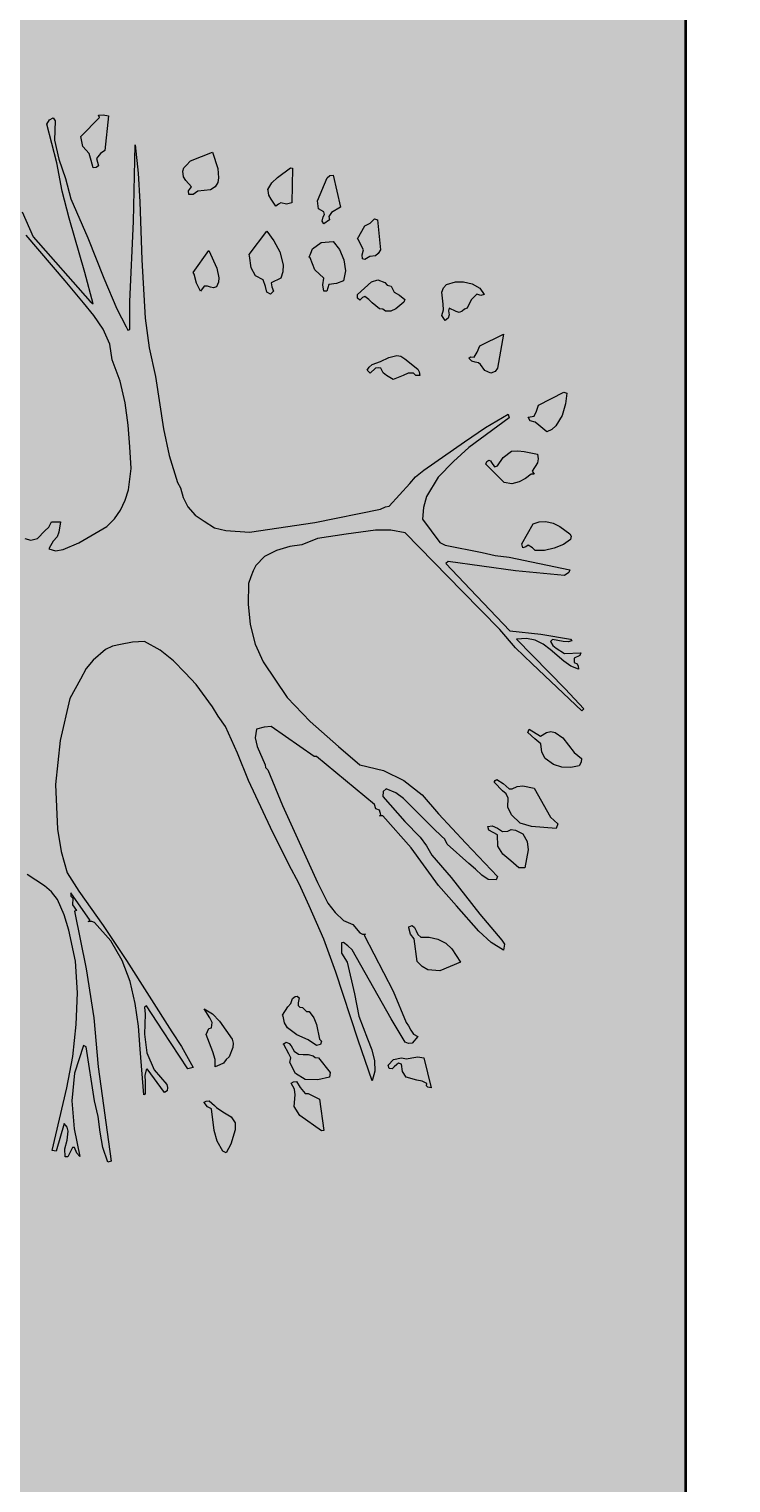
# Model space of a CAD drawing. Units: inches. Extents: x 84 to 1044, y -280 to 906.
# Tile 102 of 105: x 882 to 897, y 478 to 510. Entities that reach past the tile are written whole.
import ezdxf

# ---------------------------------------------------------------- set-up
doc = ezdxf.new("R2010")
doc.units = ezdxf.units.IN
for name, color, linetype, lineweight in [('A-ANNO-DIMS', 2, 'Continuous', 18), ('L-PLNT', 114, 'Continuous', 15), ('WALL', 250, 'Continuous', 35)]:
    doc.layers.add(name, color=color, linetype=linetype, lineweight=lineweight)
doc.layers.add('L-PLNT-PATT', color=9, linetype='Continuous', lineweight=9, true_color=0xafd9aa)
doc.styles.get("Standard").update_dxf_attribs({"font": 'arial.ttf'})
doc.dimstyles.get("Standard").update_dxf_attribs({"dimtxt": 0.18, "dimasz": 0.18, "dimexe": 0.18, "dimexo": 0.0625, "dimgap": 0.09, "dimtad": 0, "dimtih": 1, "dimtoh": 1, "dimdec": 4, "dimzin": 0, "dimdsep": 46, "dimtxsty": 'Standard', "dimcen": 0.09, "dimadec": 0, "dimazin": 0, "dimtfac": 1, "dimtdec": 4, "dimtofl": 0, "dimtmove": 0, "dimatfit": 3, "dimfxl": 1, "dimtolj": 1, "dimtzin": 0, "dimarcsym": 0})

# ---------------------------------------------------------------- blocks, each defined once
blk = doc.blocks.new('A$C37E508DF')
for p, q in [((0.7083, 1.5239), (0.7152, 1.5244)), ((0.7096, 1.5209), (0.7083, 1.5239)), ((0.7152, 1.5244), (0.7225, 1.5231)), ((0.6329, 1.5111), (0.6367, 1.5175)), ((0.6475, 1.4545), (0.6329, 1.5111)), ((0.6367, 1.5175), (0.6423, 1.5201)), ((0.6423, 1.5201), (0.6453, 1.5158)), ((0.6453, 1.5158), (0.644, 1.4879)), ((0.6826, 1.493), (0.7096, 1.5209)), ((0.7225, 1.5231), (0.7174, 1.4729)), ((0.644, 1.4879), (0.6505, 1.46)), ((0.6852, 1.4785), (0.6826, 1.493)), ((0.6946, 1.4682), (0.6852, 1.4785)), ((0.6976, 1.4579), (0.6946, 1.4682)), ((0.7109, 1.4682), (0.7053, 1.4609)), ((0.7053, 1.4609), (0.7083, 1.4502)), ((0.7174, 1.4729), (0.7109, 1.4682)), ((0.7589, 1.3691), (0.7615, 1.481)), ((0.7615, 1.481), (0.7658, 1.4395)), ((0.8421, 1.4575), (0.8739, 1.4703)), ((0.8739, 1.4703), (0.882, 1.4463)), ((0.6552, 1.4137), (0.6475, 1.4545)), ((0.6505, 1.46), (0.6603, 1.4317)), ((0.7002, 1.4476), (0.6976, 1.4579)), ((0.7049, 1.448), (0.7002, 1.4476)), ((0.7083, 1.4502), (0.7049, 1.448)), ((0.7658, 1.4395), (0.7684, 1.3979)), ((0.831, 1.4424), (0.8323, 1.4476)), ((0.8318, 1.4343), (0.831, 1.4424)), ((0.8323, 1.4476), (0.8357, 1.451)), ((0.8357, 1.451), (0.8421, 1.4575)), ((0.882, 1.4463), (0.8829, 1.433)), ((0.9686, 1.4334), (0.9875, 1.4476)), ((0.9875, 1.4476), (0.9905, 1.4467)), ((0.9905, 1.4467), (0.9896, 1.3966)), ((0.6603, 1.4317), (0.668, 1.4021)), ((0.8353, 1.4292), (0.8318, 1.4343)), ((0.8434, 1.4197), (0.8353, 1.4292)), ((0.8391, 1.4141), (0.8434, 1.4197)), ((0.8781, 1.4197), (0.8709, 1.4154)), ((0.8816, 1.4262), (0.8781, 1.4197)), ((0.8829, 1.433), (0.8816, 1.4262)), ((0.9545, 1.4159), (0.9605, 1.4257)), ((0.9605, 1.4257), (0.9686, 1.4334)), ((1.0269, 1.3996), (1.0411, 1.433)), ((1.0411, 1.433), (1.045, 1.4365)), ((1.045, 1.4365), (1.0497, 1.4369)), ((1.0497, 1.4369), (1.0604, 1.3901)), ((0.6655, 1.3743), (0.6552, 1.4137)), ((0.668, 1.4021), (0.6925, 1.3455)), ((0.7684, 1.3979), (0.771, 1.3134)), ((0.8395, 1.4086), (0.8391, 1.4141)), ((0.846, 1.4086), (0.8395, 1.4086)), ((0.8528, 1.4137), (0.846, 1.4086)), ((0.8619, 1.4146), (0.8528, 1.4137)), ((0.8709, 1.4154), (0.8619, 1.4146)), ((0.9549, 1.4146), (0.9545, 1.4159)), ((0.9558, 1.4077), (0.9549, 1.4146)), ((0.9592, 1.4017), (0.9558, 1.4077)), ((0.966, 1.3914), (0.9592, 1.4017)), ((1.0282, 1.3876), (1.0269, 1.3996)), ((0.5969, 1.3833), (0.6132, 1.3472)), ((0.9703, 1.3944), (0.966, 1.3914)), ((0.9733, 1.3966), (0.9703, 1.3944)), ((0.9819, 1.3944), (0.9733, 1.3966)), ((0.9896, 1.3966), (0.9819, 1.3944)), ((1.0359, 1.3833), (1.0282, 1.3876)), ((1.0334, 1.37), (1.0351, 1.376)), ((1.0351, 1.376), (1.0368, 1.3794)), ((1.0368, 1.3794), (1.0359, 1.3833)), ((1.0471, 1.3824), (1.0432, 1.3764)), ((1.0432, 1.3764), (1.0441, 1.3717)), ((1.0604, 1.3901), (1.0471, 1.3824)), ((0.6882, 1.2949), (0.6655, 1.3743)), ((0.7538, 1.2529), (0.7589, 1.3691)), ((0.9274, 1.3215), (0.9532, 1.3554)), ((0.9532, 1.3554), (0.9635, 1.3413)), ((1.0359, 1.3661), (1.0334, 1.37)), ((1.0441, 1.3717), (1.0359, 1.3661)), ((1.0848, 1.3443), (1.0955, 1.3631)), ((1.0955, 1.3631), (1.1033, 1.367)), ((1.1033, 1.367), (1.1097, 1.373)), ((1.1097, 1.373), (1.114, 1.3717)), ((1.114, 1.3717), (1.1183, 1.328)), ((0.6595, 1.2829), (0.6029, 1.3494)), ((0.6132, 1.3472), (0.6959, 1.2529)), ((0.6925, 1.3455), (0.7161, 1.2868)), ((0.9635, 1.3413), (0.9721, 1.325)), ((1.0197, 1.3297), (1.0321, 1.3387)), ((1.0321, 1.3387), (1.0497, 1.3404)), ((1.0497, 1.3404), (1.0587, 1.3284)), ((1.0861, 1.343), (1.0848, 1.3443)), ((1.0938, 1.328), (1.0861, 1.343)), ((0.771, 1.3134), (0.7761, 1.2285)), ((0.846, 1.2949), (0.8687, 1.3271)), ((0.8687, 1.3271), (0.8803, 1.3014)), ((0.9279, 1.3194), (0.9274, 1.3215)), ((0.9305, 1.3018), (0.9279, 1.3194)), ((0.9721, 1.325), (0.9768, 1.3061)), ((1.0149, 1.3172), (1.0171, 1.3232)), ((1.0162, 1.3164), (1.0149, 1.3172)), ((1.0231, 1.2988), (1.0162, 1.3164)), ((1.0171, 1.3232), (1.0197, 1.3297)), ((1.0587, 1.3284), (1.0651, 1.3134)), ((1.0651, 1.3134), (1.0677, 1.2975)), ((1.0917, 1.3207), (1.0938, 1.328)), ((1.0925, 1.3151), (1.0917, 1.3207)), ((1.0955, 1.3138), (1.0925, 1.3151)), ((1.1028, 1.3185), (1.0955, 1.3138)), ((1.111, 1.3194), (1.1028, 1.3185)), ((1.1153, 1.3228), (1.111, 1.3194)), ((1.1183, 1.328), (1.1153, 1.3228)), ((0.7002, 1.2495), (0.6882, 1.2949)), ((0.8473, 1.2924), (0.846, 1.2949)), ((0.8507, 1.2795), (0.8473, 1.2924)), ((0.8803, 1.3014), (0.8833, 1.2872)), ((0.9365, 1.2902), (0.9305, 1.3018)), ((0.9763, 1.2962), (0.9733, 1.2868)), ((0.9768, 1.3061), (0.9763, 1.2962)), ((1.0359, 1.2868), (1.0231, 1.2988)), ((1.0677, 1.2975), (1.0647, 1.2829)), ((0.6865, 1.2508), (0.6595, 1.2829)), ((0.7161, 1.2868), (0.7349, 1.2422)), ((0.8567, 1.2679), (0.8507, 1.2795)), ((0.8619, 1.2752), (0.8567, 1.2679)), ((0.867, 1.2752), (0.8619, 1.2752)), ((0.8713, 1.2739), (0.867, 1.2752)), ((0.8756, 1.2726), (0.8713, 1.2739)), ((0.8799, 1.2744), (0.8756, 1.2726)), ((0.8829, 1.2808), (0.8799, 1.2744)), ((0.8833, 1.2872), (0.8829, 1.2808)), ((0.9476, 1.2842), (0.9365, 1.2902)), ((0.951, 1.2748), (0.9476, 1.2842)), ((0.9532, 1.2666), (0.951, 1.2748)), ((0.9733, 1.2868), (0.9596, 1.2799)), ((0.9596, 1.2799), (0.9605, 1.2744)), ((0.9605, 1.2744), (0.9626, 1.2679)), ((1.0347, 1.2769), (1.0359, 1.2868)), ((1.0359, 1.2679), (1.0347, 1.2769)), ((1.0432, 1.2774), (1.0402, 1.2679)), ((1.0544, 1.2791), (1.0432, 1.2774)), ((1.0647, 1.2829), (1.0544, 1.2791)), ((1.0848, 1.2628), (1.1054, 1.2817)), ((1.1054, 1.2817), (1.1148, 1.2842)), ((1.1148, 1.2842), (1.1247, 1.2804)), ((1.1247, 1.2804), (1.1281, 1.2765)), ((1.1281, 1.2765), (1.1341, 1.2752)), ((1.1341, 1.2752), (1.1384, 1.2666)), ((1.2075, 1.2666), (1.21, 1.2726)), ((1.21, 1.2726), (1.2147, 1.2774)), ((1.2147, 1.2774), (1.2276, 1.2817)), ((1.2276, 1.2817), (1.2392, 1.2817)), ((1.2392, 1.2817), (1.2521, 1.2787)), ((1.2521, 1.2787), (1.2632, 1.2722)), ((1.2632, 1.2722), (1.2692, 1.2628)), ((0.7015, 1.2323), (0.6865, 1.2508)), ((0.6959, 1.2529), (0.7002, 1.2495)), ((0.7538, 1.2122), (0.7538, 1.2529)), ((0.9583, 1.2636), (0.9532, 1.2666)), ((0.9626, 1.2679), (0.9583, 1.2636)), ((1.0402, 1.2679), (1.0359, 1.2679)), ((1.0852, 1.2576), (1.0848, 1.2628)), ((1.0883, 1.2546), (1.0852, 1.2576)), ((1.0921, 1.2585), (1.0883, 1.2546)), ((1.0955, 1.2602), (1.0921, 1.2585)), ((1.1015, 1.2559), (1.0955, 1.2602)), ((1.1063, 1.2508), (1.1015, 1.2559)), ((1.117, 1.2422), (1.1063, 1.2508)), ((1.1384, 1.2666), (1.1461, 1.2619)), ((1.1526, 1.2521), (1.141, 1.2422)), ((1.1461, 1.2619), (1.1539, 1.2559)), ((1.1539, 1.2559), (1.1526, 1.2521)), ((1.2096, 1.2491), (1.2075, 1.2666)), ((1.21, 1.2409), (1.2096, 1.2491)), ((1.2503, 1.2551), (1.2448, 1.2431)), ((1.2585, 1.2636), (1.2503, 1.2551)), ((1.2645, 1.2615), (1.2585, 1.2636)), ((1.2692, 1.2628), (1.2645, 1.2615)), ((0.7148, 1.2126), (0.7015, 1.2323)), ((0.7349, 1.2422), (0.7482, 1.216)), ((0.7761, 1.2285), (0.7821, 1.1856)), ((1.1221, 1.2418), (1.117, 1.2422)), ((1.126, 1.2388), (1.1221, 1.2418)), ((1.1337, 1.2388), (1.126, 1.2388)), ((1.141, 1.2422), (1.1337, 1.2388)), ((1.2079, 1.2323), (1.21, 1.2409)), ((1.2126, 1.2251), (1.2079, 1.2323)), ((1.2169, 1.2285), (1.2126, 1.2251)), ((1.2186, 1.2332), (1.2169, 1.2285)), ((1.2186, 1.2431), (1.2173, 1.2392)), ((1.2173, 1.2392), (1.2186, 1.2332)), ((1.2285, 1.2383), (1.2186, 1.2431)), ((1.2328, 1.2366), (1.2285, 1.2383)), ((1.2371, 1.2388), (1.2328, 1.2366)), ((1.2405, 1.2418), (1.2371, 1.2388)), ((1.2448, 1.2431), (1.2405, 1.2418)), ((0.7246, 1.1908), (0.7148, 1.2126)), ((0.7482, 1.216), (0.7508, 1.2109)), ((0.7508, 1.2109), (0.7538, 1.2122)), ((0.7281, 1.168), (0.7246, 1.1908)), ((0.7821, 1.1856), (0.7911, 1.1436)), ((1.2589, 1.1792), (1.2628, 1.1882)), ((1.2628, 1.1882), (1.2975, 1.2053)), ((1.2975, 1.2053), (1.2885, 1.1556)), ((0.7396, 1.1371), (0.7281, 1.168)), ((1.1063, 1.1612), (1.1187, 1.1655)), ((1.1187, 1.1655), (1.1307, 1.1714)), ((1.1307, 1.1714), (1.1423, 1.1744)), ((1.1423, 1.1744), (1.1483, 1.1732)), ((1.1483, 1.1732), (1.1539, 1.1693)), ((1.1539, 1.1693), (1.1727, 1.1543)), ((1.2469, 1.1702), (1.2495, 1.1723)), ((1.2478, 1.1693), (1.2469, 1.1702)), ((1.2516, 1.1659), (1.2478, 1.1693)), ((1.2495, 1.1723), (1.2546, 1.1719)), ((1.2563, 1.1646), (1.2516, 1.1659)), ((1.2546, 1.1719), (1.2589, 1.1792)), ((1.2611, 1.1637), (1.2563, 1.1646)), ((0.7911, 1.1436), (0.8027, 1.0677)), ((1.099, 1.153), (1.102, 1.1573)), ((1.1033, 1.1487), (1.099, 1.153)), ((1.102, 1.1573), (1.1063, 1.1612)), ((1.111, 1.156), (1.1033, 1.1487)), ((1.1153, 1.1564), (1.111, 1.156)), ((1.1191, 1.1556), (1.1153, 1.1564)), ((1.1226, 1.1492), (1.1191, 1.1556)), ((1.1273, 1.1453), (1.1226, 1.1492)), ((1.1367, 1.1393), (1.1273, 1.1453)), ((1.1517, 1.1453), (1.1367, 1.1393)), ((1.1586, 1.1483), (1.1517, 1.1453)), ((1.1663, 1.1487), (1.1586, 1.1483)), ((1.1697, 1.1449), (1.1663, 1.1487)), ((1.1757, 1.1449), (1.1697, 1.1449)), ((1.1727, 1.1543), (1.1749, 1.1504)), ((1.1749, 1.1504), (1.1757, 1.1449)), ((1.2641, 1.1612), (1.2611, 1.1637)), ((1.2701, 1.1522), (1.2641, 1.1612)), ((1.2791, 1.1487), (1.2701, 1.1522)), ((1.2851, 1.1509), (1.2791, 1.1487)), ((1.2885, 1.1556), (1.2851, 1.1509)), ((0.7469, 1.1054), (0.7396, 1.1371)), ((0.7512, 1.0728), (0.7469, 1.1054)), ((1.3455, 1.0934), (1.3485, 1.102)), ((1.3485, 1.102), (1.385, 1.1209)), ((1.3875, 1.1037), (1.3828, 1.087)), ((1.385, 1.1209), (1.3897, 1.1196)), ((1.3897, 1.1196), (1.3875, 1.1037)), ((1.3057, 1.0835), (1.2469, 1.0402)), ((1.2713, 1.0694), (1.3044, 1.0887)), ((1.3044, 1.0887), (1.3057, 1.0835)), ((1.3335, 1.0844), (1.3421, 1.0861)), ((1.3361, 1.0793), (1.3335, 1.0844)), ((1.3421, 1.0861), (1.3455, 1.0934)), ((1.3828, 1.087), (1.3738, 1.072)), ((0.7538, 1.0415), (0.7512, 1.0728)), ((0.8027, 1.0677), (0.8108, 1.0287)), ((1.2409, 1.0488), (1.2713, 1.0694)), ((1.3434, 1.0771), (1.3361, 1.0793)), ((1.349, 1.0728), (1.3434, 1.0771)), ((1.3605, 1.063), (1.349, 1.0728)), ((1.3678, 1.0664), (1.3605, 1.063)), ((1.3738, 1.072), (1.3678, 1.0664)), ((0.7559, 1.0098), (0.7538, 1.0415)), ((1.1813, 1.0072), (1.2409, 1.0488)), ((1.2469, 1.0402), (1.2246, 1.0201)), ((0.8108, 1.0287), (0.8233, 0.9892)), ((1.2246, 1.0201), (1.2023, 0.9969)), ((1.2718, 1.0162), (1.2731, 1.0197)), ((1.2984, 0.9892), (1.2718, 1.0162)), ((1.2731, 1.0197), (1.2761, 1.0218)), ((1.2761, 1.0218), (1.2786, 1.0209)), ((1.2786, 1.0209), (1.2799, 1.0184)), ((1.2799, 1.0184), (1.2842, 1.0124)), ((1.2885, 1.0136), (1.2971, 1.0257)), ((1.2971, 1.0257), (1.3091, 1.0351)), ((1.3091, 1.0351), (1.3185, 1.0355)), ((1.3185, 1.0355), (1.3275, 1.0347)), ((1.3275, 1.0347), (1.3468, 1.0308)), ((1.3468, 1.018), (1.3391, 1.0059)), ((1.3468, 1.0308), (1.3481, 1.0239)), ((1.3481, 1.0239), (1.3468, 1.018)), ((0.7516, 0.9785), (0.7559, 1.0098)), ((1.1612, 0.9879), (1.1693, 0.9974)), ((1.1693, 0.9974), (1.1813, 1.0072)), ((1.2023, 0.9969), (1.1852, 0.9691)), ((1.2842, 1.0124), (1.2885, 1.0136)), ((1.3297, 0.9952), (1.3202, 0.9901)), ((1.3378, 1.0016), (1.3297, 0.9952)), ((1.3421, 1.0016), (1.3378, 1.0016)), ((1.3391, 1.0059), (1.3421, 1.0016)), ((0.7469, 0.9635), (0.7516, 0.9785)), ((0.8233, 0.9892), (0.8275, 0.9815)), ((0.8275, 0.9815), (0.8314, 0.9673)), ((1.1311, 0.9549), (1.1612, 0.9879)), ((1.3095, 0.9875), (1.2984, 0.9892)), ((1.3202, 0.9901), (1.3095, 0.9875)), ((0.7401, 0.9493), (0.7469, 0.9635)), ((0.8314, 0.9673), (0.8383, 0.954)), ((0.8383, 0.954), (0.8486, 0.942)), ((1.1183, 0.9506), (1.1256, 0.954)), ((1.1256, 0.954), (1.1311, 0.9549)), ((1.1809, 0.9532), (1.1796, 0.936)), ((1.1852, 0.9691), (1.1809, 0.9532)), ((0.6359, 0.9245), (0.6397, 0.9322)), ((0.6397, 0.9322), (0.653, 0.9322)), ((0.653, 0.9322), (0.6505, 0.9172)), ((0.7203, 0.9253), (0.7315, 0.9365)), ((0.7315, 0.9365), (0.7401, 0.9493)), ((0.8486, 0.942), (0.8619, 0.933)), ((0.8619, 0.933), (0.8769, 0.9236)), ((1.0227, 0.9309), (1.1183, 0.9506)), ((1.1796, 0.936), (1.2049, 0.9022)), ((1.3404, 0.9292), (1.3494, 0.9322)), ((1.3494, 0.9322), (1.3592, 0.9326)), ((1.3592, 0.9326), (1.3695, 0.93)), ((0.6196, 0.9077), (0.6303, 0.9189)), ((0.6303, 0.9189), (0.6359, 0.9245)), ((0.6479, 0.9103), (0.6423, 0.9039)), ((0.6505, 0.9172), (0.6479, 0.9103)), ((0.6796, 0.9013), (0.7203, 0.9253)), ((0.8769, 0.9236), (0.8936, 0.9193)), ((0.8936, 0.9193), (0.9279, 0.9172)), ((0.9279, 0.9172), (1.0227, 0.9309)), ((1.0685, 0.9142), (1.0269, 0.9077)), ((1.1114, 0.9198), (1.0685, 0.9142)), ((1.1333, 0.9202), (1.1114, 0.9198)), ((1.1543, 0.9159), (1.1333, 0.9202)), ((1.2371, 0.8314), (1.1543, 0.9159)), ((1.3241, 0.9), (1.3404, 0.9292)), ((1.3695, 0.93), (1.3794, 0.9253)), ((1.3794, 0.9253), (1.394, 0.9146)), ((1.394, 0.9146), (1.3957, 0.9112)), ((1.3957, 0.9112), (1.3948, 0.9065)), ((0.6011, 0.9077), (0.6097, 0.9056)), ((0.6097, 0.9056), (0.6196, 0.9077)), ((0.6384, 0.8974), (0.6359, 0.8927)), ((0.6359, 0.8927), (0.6457, 0.8897)), ((0.6423, 0.9039), (0.6384, 0.8974)), ((0.6457, 0.8897), (0.6569, 0.8919)), ((0.6569, 0.8919), (0.6796, 0.9013)), ((0.9673, 0.8906), (0.9498, 0.8816)), ((0.9866, 0.8962), (0.9673, 0.8906)), ((1.0042, 0.8987), (0.9866, 0.8962)), ((1.0269, 0.9077), (1.0042, 0.8987)), ((1.2049, 0.9022), (1.2126, 0.8983)), ((1.2126, 0.8983), (1.2662, 0.8876)), ((1.3254, 0.8944), (1.3241, 0.9)), ((1.3301, 0.8957), (1.3254, 0.8944)), ((1.3335, 0.8983), (1.3301, 0.8957)), ((1.3395, 0.8944), (1.3335, 0.8983)), ((1.3434, 0.8906), (1.3395, 0.8944)), ((1.3571, 0.8906), (1.3434, 0.8906)), ((1.3713, 0.8936), (1.3571, 0.8906)), ((1.3846, 0.8992), (1.3713, 0.8936)), ((1.3948, 0.9065), (1.3846, 0.8992)), ((0.9369, 0.8687), (0.933, 0.861)), ((0.9498, 0.8816), (0.9369, 0.8687)), ((1.2169, 0.8743), (1.2135, 0.8713)), ((1.2135, 0.8713), (1.2491, 0.834)), ((1.3151, 0.8606), (1.2169, 0.8743)), ((1.2662, 0.8876), (1.2855, 0.8833)), ((1.2855, 0.8833), (1.3057, 0.8807)), ((1.3057, 0.8807), (1.394, 0.8623)), ((0.9296, 0.852), (0.9262, 0.8421)), ((0.933, 0.861), (0.9296, 0.852)), ((1.3863, 0.8541), (1.3151, 0.8606)), ((1.3927, 0.8584), (1.3863, 0.8541)), ((1.394, 0.8623), (1.3927, 0.8584)), ((0.9262, 0.8421), (0.9257, 0.8121)), ((1.2919, 0.7752), (1.2371, 0.8314)), ((1.2491, 0.834), (1.3069, 0.7735)), ((0.9257, 0.8121), (0.9287, 0.7825)), ((0.9287, 0.7825), (0.936, 0.7542)), ((1.3151, 0.7487), (1.2919, 0.7752)), ((1.3069, 0.7735), (1.352, 0.7684)), ((1.3309, 0.7624), (1.3164, 0.7615)), ((1.3434, 0.7598), (1.3309, 0.7624)), ((1.352, 0.7684), (1.3948, 0.7615)), ((0.7182, 0.7461), (0.7002, 0.7307)), ((0.7285, 0.7512), (0.7182, 0.7461)), ((0.7401, 0.7534), (0.7285, 0.7512)), ((0.7577, 0.7568), (0.7401, 0.7534)), ((0.7752, 0.7577), (0.7577, 0.7568)), ((0.798, 0.7452), (0.7752, 0.7577)), ((0.8173, 0.7298), (0.798, 0.7452)), ((0.936, 0.7542), (0.9476, 0.7285)), ((1.3391, 0.7255), (1.3151, 0.7487)), ((1.3164, 0.7615), (1.3871, 0.6891)), ((1.355, 0.7538), (1.3434, 0.7598)), ((1.3653, 0.7461), (1.355, 0.7538)), ((1.3854, 0.7294), (1.3653, 0.7461)), ((1.3687, 0.7607), (1.3657, 0.7577)), ((1.3657, 0.7577), (1.3691, 0.7521)), ((1.3841, 0.7577), (1.3687, 0.7607)), ((1.3691, 0.7521), (1.3743, 0.7482)), ((1.3743, 0.7482), (1.3863, 0.7405)), ((1.3914, 0.7572), (1.3841, 0.7577)), ((1.3863, 0.7405), (1.4099, 0.7414)), ((1.397, 0.759), (1.3914, 0.7572)), ((1.3948, 0.7615), (1.397, 0.759)), ((1.4099, 0.7414), (1.4086, 0.7375)), ((0.7002, 0.7307), (0.6903, 0.7186)), ((0.8344, 0.7122), (0.8173, 0.7298)), ((0.9476, 0.7285), (0.9828, 0.6762)), ((1.4116, 0.6569), (1.3391, 0.7255)), ((1.3953, 0.7221), (1.3854, 0.7294)), ((1.4064, 0.7178), (1.3953, 0.7221)), ((1.4086, 0.7375), (1.4004, 0.7337)), ((1.4004, 0.7337), (1.4004, 0.7272)), ((1.4004, 0.7272), (1.4047, 0.7255)), ((1.4047, 0.7255), (1.406, 0.7221)), ((1.406, 0.7221), (1.4064, 0.7178)), ((0.6818, 0.7032), (0.6667, 0.6749)), ((0.6903, 0.7186), (0.6818, 0.7032)), ((0.8503, 0.6951), (0.8344, 0.7122)), ((0.8739, 0.6629), (0.8503, 0.6951)), ((1.3871, 0.6891), (1.4141, 0.6599)), ((0.6667, 0.6749), (0.6526, 0.614)), ((0.8824, 0.6492), (0.8739, 0.6629)), ((0.9828, 0.6762), (1.0162, 0.6415)), ((1.4141, 0.6599), (1.4116, 0.6569)), ((0.8932, 0.6342), (0.8824, 0.6492)), ((1.0162, 0.6415), (1.0574, 0.605)), ((0.6526, 0.614), (0.6457, 0.5497)), ((0.9103, 0.5956), (0.8932, 0.6342)), ((0.9382, 0.6303), (0.936, 0.6179)), ((0.936, 0.6179), (0.939, 0.605)), ((0.9493, 0.6333), (0.9382, 0.6303)), ((0.9596, 0.6342), (0.9493, 0.6333)), ((1.0218, 0.5904), (0.9596, 0.6342)), ((1.3327, 0.6252), (1.3348, 0.6303)), ((1.343, 0.6162), (1.3327, 0.6252)), ((1.3348, 0.6303), (1.3511, 0.62)), ((1.352, 0.6089), (1.343, 0.6162)), ((1.3511, 0.62), (1.3601, 0.6256)), ((1.3601, 0.6256), (1.3661, 0.6269)), ((1.3661, 0.6269), (1.3725, 0.6252)), ((1.3725, 0.6252), (1.3837, 0.6175)), ((1.3837, 0.6175), (1.3918, 0.6072)), ((0.9262, 0.5557), (0.9103, 0.5956)), ((0.939, 0.605), (0.9506, 0.5784)), ((1.0574, 0.605), (1.0883, 0.5784)), ((1.3533, 0.5969), (1.352, 0.6089)), ((1.358, 0.5874), (1.3533, 0.5969)), ((1.3918, 0.6072), (1.4004, 0.5964)), ((1.4004, 0.5964), (1.4111, 0.5874)), ((0.9506, 0.5784), (0.951, 0.5746)), ((0.951, 0.5746), (0.9545, 0.5711)), ((1.0256, 0.5904), (1.0218, 0.5904)), ((1.1097, 0.5205), (1.0256, 0.5904)), ((1.0883, 0.5784), (1.123, 0.5703)), ((1.37, 0.5789), (1.358, 0.5874)), ((1.3824, 0.575), (1.37, 0.5789)), ((1.3953, 0.5746), (1.3824, 0.575)), ((1.4077, 0.5771), (1.3953, 0.5746)), ((1.4103, 0.5823), (1.4077, 0.5771)), ((1.4111, 0.5874), (1.4103, 0.5823)), ((0.9583, 0.4871), (0.9262, 0.5557)), ((0.9545, 0.5711), (0.9759, 0.5193)), ((1.123, 0.5703), (1.1526, 0.5557)), ((1.1526, 0.5557), (1.1792, 0.5347)), ((1.2842, 0.554), (1.2855, 0.5557)), ((1.2842, 0.5527), (1.2842, 0.554)), ((1.2958, 0.5407), (1.2842, 0.5527)), ((1.2855, 0.5557), (1.2876, 0.557)), ((1.2876, 0.557), (1.2971, 0.551)), ((1.2971, 0.551), (1.3057, 0.5433)), ((0.6457, 0.5497), (0.6483, 0.4845)), ((1.1226, 0.5394), (1.1221, 0.5325)), ((1.1221, 0.5325), (1.1539, 0.4961)), ((1.1268, 0.5433), (1.1226, 0.5394)), ((1.141, 0.5377), (1.1268, 0.5433)), ((1.1521, 0.5296), (1.141, 0.5377)), ((1.1706, 0.5111), (1.1521, 0.5296)), ((1.1792, 0.5347), (1.2027, 0.5072)), ((1.3014, 0.536), (1.2958, 0.5407)), ((1.3044, 0.53), (1.3014, 0.536)), ((1.3039, 0.5167), (1.3044, 0.53)), ((1.3057, 0.5433), (1.3099, 0.5433)), ((1.3099, 0.5433), (1.3172, 0.5467)), ((1.3172, 0.5467), (1.3254, 0.548)), ((1.3254, 0.548), (1.3421, 0.5446)), ((1.3421, 0.5446), (1.3657, 0.5021)), ((0.9759, 0.5193), (1.0269, 0.4069)), ((1.1118, 0.5145), (1.1097, 0.5205)), ((1.117, 0.5124), (1.1118, 0.5145)), ((1.1191, 0.5055), (1.117, 0.5124)), ((1.1955, 0.4858), (1.1706, 0.5111)), ((1.3091, 0.5055), (1.3039, 0.5167)), ((0.9853, 0.4335), (0.9583, 0.4871)), ((1.117, 0.5042), (1.1191, 0.5055)), ((1.1217, 0.5042), (1.117, 0.5042)), ((1.1633, 0.4575), (1.1217, 0.5042)), ((1.1539, 0.4961), (1.1762, 0.4729)), ((1.2027, 0.5072), (1.2426, 0.4644)), ((1.2748, 0.4884), (1.2812, 0.4897)), ((1.2761, 0.4832), (1.2748, 0.4884)), ((1.2812, 0.4897), (1.2885, 0.4862)), ((1.3215, 0.4935), (1.3091, 0.5055)), ((1.3382, 0.4884), (1.3215, 0.4935)), ((1.3743, 0.4858), (1.3382, 0.4884)), ((1.3657, 0.5021), (1.3764, 0.4927)), ((1.3764, 0.4927), (1.3743, 0.4858)), ((0.6483, 0.4845), (0.6539, 0.4524)), ((1.1762, 0.4729), (1.1856, 0.4605)), ((1.207, 0.4747), (1.1955, 0.4858)), ((1.2122, 0.47), (1.207, 0.4747)), ((1.2156, 0.4627), (1.2122, 0.47)), ((1.2825, 0.4798), (1.2761, 0.4832)), ((1.2885, 0.4764), (1.2825, 0.4798)), ((1.2885, 0.4862), (1.2962, 0.4815)), ((1.2894, 0.4601), (1.2885, 0.4764)), ((1.2962, 0.4815), (1.3039, 0.482)), ((1.3039, 0.482), (1.3087, 0.4841)), ((1.3087, 0.4841), (1.3147, 0.4832)), ((1.3147, 0.4832), (1.3258, 0.4777)), ((1.3258, 0.4777), (1.3318, 0.4669)), ((1.3318, 0.4669), (1.3331, 0.4545)), ((0.6539, 0.4524), (0.6625, 0.4211)), ((1.2027, 0.4026), (1.1633, 0.4575)), ((1.1856, 0.4605), (1.1933, 0.4468)), ((1.1933, 0.4468), (1.2212, 0.4146)), ((1.2469, 0.4348), (1.2156, 0.4627)), ((1.2426, 0.4644), (1.2885, 0.4159)), ((1.2967, 0.4485), (1.2894, 0.4601)), ((1.3082, 0.4386), (1.2967, 0.4485)), ((1.3331, 0.4545), (1.3284, 0.4284)), ((1.0003, 0.4052), (0.9853, 0.4335)), ((1.2568, 0.4266), (1.2469, 0.4348)), ((1.2658, 0.4176), (1.2568, 0.4266)), ((1.3198, 0.4284), (1.3082, 0.4386)), ((1.3284, 0.4284), (1.3198, 0.4284)), ((0.6295, 0.4022), (0.6046, 0.4189)), ((0.6397, 0.3936), (0.6295, 0.4022)), ((0.6625, 0.4211), (0.6796, 0.3945)), ((1.0145, 0.373), (1.0003, 0.4052)), ((1.0269, 0.4069), (1.0419, 0.3769)), ((1.2289, 0.373), (1.2027, 0.4026)), ((1.2212, 0.4146), (1.2628, 0.361)), ((1.2752, 0.4116), (1.2658, 0.4176)), ((1.2868, 0.4108), (1.2752, 0.4116)), ((1.2885, 0.4159), (1.2868, 0.4108)), ((0.6487, 0.3825), (0.6397, 0.3936)), ((0.6582, 0.3602), (0.6487, 0.3825)), ((0.6959, 0.352), (0.668, 0.3919)), ((0.668, 0.3919), (0.668, 0.3872)), ((0.668, 0.3872), (0.6706, 0.3842)), ((0.6706, 0.3842), (0.6702, 0.3748)), ((0.6796, 0.3945), (0.7148, 0.3447)), ((0.665, 0.3379), (0.6582, 0.3602)), ((0.6702, 0.3748), (0.6762, 0.3662)), ((0.6762, 0.3662), (0.6732, 0.3653)), ((0.6732, 0.3653), (0.6903, 0.2813)), ((1.0359, 0.3246), (1.0145, 0.373)), ((1.0419, 0.3769), (1.0527, 0.3632)), ((1.0527, 0.3632), (1.0647, 0.352)), ((1.2615, 0.3362), (1.2289, 0.373)), ((1.2628, 0.361), (1.2949, 0.3233)), ((0.6933, 0.3503), (0.6959, 0.352)), ((0.6985, 0.3503), (0.6933, 0.3503)), ((0.7023, 0.349), (0.6985, 0.3503)), ((0.7259, 0.3224), (0.7023, 0.349)), ((0.7148, 0.3447), (0.7487, 0.2937)), ((1.0647, 0.352), (1.078, 0.346)), ((1.078, 0.346), (1.0883, 0.334)), ((1.1599, 0.3426), (1.1646, 0.3447)), ((1.1599, 0.3413), (1.1599, 0.3426)), ((1.162, 0.3319), (1.1599, 0.3413)), ((1.1646, 0.3447), (1.168, 0.3417)), ((1.168, 0.3417), (1.1702, 0.3366)), ((0.6745, 0.2924), (0.665, 0.3379)), ((0.7427, 0.2937), (0.7259, 0.3224)), ((1.0535, 0.2766), (1.0359, 0.3246)), ((1.0647, 0.3199), (1.0617, 0.3194)), ((1.0617, 0.3194), (1.0617, 0.304)), ((1.0711, 0.3147), (1.0647, 0.3199)), ((1.0883, 0.334), (1.0921, 0.3319)), ((1.0921, 0.3319), (1.0968, 0.3319)), ((1.0968, 0.3319), (1.0947, 0.3306)), ((1.0947, 0.3306), (1.1367, 0.2491)), ((1.1676, 0.325), (1.162, 0.3319)), ((1.1719, 0.292), (1.1676, 0.325)), ((1.1702, 0.3366), (1.1727, 0.3314)), ((1.1727, 0.3314), (1.177, 0.3276)), ((1.177, 0.3276), (1.1895, 0.3276)), ((1.1895, 0.3276), (1.2019, 0.3246)), ((1.2019, 0.3246), (1.2135, 0.3186)), ((1.2135, 0.3186), (1.2225, 0.3104)), ((1.2795, 0.3199), (1.2615, 0.3362)), ((1.2975, 0.3087), (1.2795, 0.3199)), ((1.2949, 0.3233), (1.2988, 0.3173)), ((1.0617, 0.304), (1.0698, 0.2911)), ((1.0775, 0.3092), (1.0711, 0.3147)), ((1.1341, 0.2084), (1.0775, 0.3092)), ((1.2225, 0.3104), (1.2349, 0.2911)), ((1.2988, 0.3173), (1.2975, 0.3087)), ((0.6775, 0.2465), (0.6745, 0.2924)), ((0.6903, 0.2813), (0.7015, 0.2101)), ((0.7542, 0.2628), (0.7427, 0.2937)), ((0.7487, 0.2937), (0.8151, 0.1899)), ((1.0861, 0.1775), (1.0535, 0.2766)), ((1.0698, 0.2911), (1.0805, 0.2448)), ((1.1792, 0.2847), (1.1719, 0.292)), ((1.1873, 0.28), (1.1792, 0.2847)), ((1.2049, 0.2783), (1.1873, 0.28)), ((1.2349, 0.2911), (1.2049, 0.2783)), ((0.7615, 0.2311), (0.7542, 0.2628)), ((0.6758, 0.2002), (0.6775, 0.2465)), ((0.9879, 0.2311), (0.9905, 0.2384)), ((0.9905, 0.2384), (0.9943, 0.241)), ((0.9943, 0.241), (0.9973, 0.2414)), ((0.9973, 0.2414), (1.0003, 0.2393)), ((1.0003, 0.2393), (0.9986, 0.232)), ((1.0805, 0.2448), (1.087, 0.2127)), ((1.1367, 0.2491), (1.1556, 0.2032)), ((0.7662, 0.1981), (0.7615, 0.2311)), ((0.7778, 0.2277), (0.7752, 0.2255)), ((0.7752, 0.2255), (0.7761, 0.2152)), ((0.7761, 0.2152), (0.7752, 0.1861)), ((0.8018, 0.1912), (0.7778, 0.2277)), ((0.8619, 0.2234), (0.8739, 0.2161)), ((0.87, 0.2101), (0.8619, 0.2234)), ((0.8739, 0.2161), (0.8841, 0.2054)), ((0.9759, 0.214), (0.9836, 0.226)), ((0.9768, 0.2127), (0.9759, 0.214)), ((0.9789, 0.2028), (0.9768, 0.2127)), ((0.9836, 0.226), (0.9879, 0.2311)), ((0.9986, 0.232), (0.9986, 0.2281)), ((0.9986, 0.2281), (1.0012, 0.2255)), ((1.0012, 0.2255), (1.0051, 0.2251)), ((1.0051, 0.2251), (1.0076, 0.2225)), ((1.0076, 0.2225), (1.0106, 0.2195)), ((1.0106, 0.2195), (1.0149, 0.2191)), ((1.0149, 0.2191), (1.0214, 0.2101)), ((1.087, 0.2127), (1.0998, 0.1797)), ((0.6706, 0.1539), (0.6758, 0.2002)), ((0.7015, 0.2101), (0.7079, 0.1389)), ((0.7688, 0.1646), (0.7662, 0.1981)), ((0.8383, 0.1359), (0.8018, 0.1912)), ((0.8649, 0.1857), (0.8687, 0.1947)), ((0.8687, 0.1947), (0.8726, 0.1955)), ((0.8734, 0.2032), (0.87, 0.2101)), ((0.8726, 0.1955), (0.8734, 0.2032)), ((0.8841, 0.2054), (0.9026, 0.1792)), ((0.9832, 0.1955), (0.9789, 0.2028)), ((0.9969, 0.1852), (0.9832, 0.1955)), ((1.0214, 0.2101), (1.0252, 0.2002)), ((1.0252, 0.2002), (1.0295, 0.1788)), ((1.1543, 0.1749), (1.1341, 0.2084)), ((1.1556, 0.2032), (1.1594, 0.1985)), ((1.1594, 0.1985), (1.1624, 0.1921)), ((1.1624, 0.1921), (1.1663, 0.1861)), ((0.6865, 0.1698), (0.6732, 0.1295)), ((0.6903, 0.1681), (0.6865, 0.1698)), ((0.7752, 0.1861), (0.7787, 0.1591)), ((0.8151, 0.1899), (0.8288, 0.1685)), ((0.8743, 0.1608), (0.8649, 0.1857)), ((0.9026, 0.1792), (0.9043, 0.1732)), ((0.9043, 0.1732), (0.9035, 0.1668)), ((0.9768, 0.1719), (0.9811, 0.1749)), ((0.9776, 0.1711), (0.9768, 0.1719)), ((0.9853, 0.1578), (0.9776, 0.1711)), ((0.9811, 0.1749), (0.9858, 0.1728)), ((0.9858, 0.1728), (0.9884, 0.1694)), ((0.9884, 0.1694), (0.9931, 0.1616)), ((1.0132, 0.1779), (0.9969, 0.1852)), ((1.0256, 0.1698), (1.0132, 0.1779)), ((1.0312, 0.1711), (1.0256, 0.1698)), ((1.0295, 0.1788), (1.0325, 0.1762)), ((1.0325, 0.1762), (1.0312, 0.1711)), ((1.1063, 0.1183), (1.0861, 0.1775)), ((1.0998, 0.1797), (1.1058, 0.1634)), ((1.1594, 0.1728), (1.1543, 0.1749)), ((1.1646, 0.1732), (1.1594, 0.1728)), ((1.1727, 0.1827), (1.1646, 0.1732)), ((1.1663, 0.1861), (1.1727, 0.1827)), ((0.662, 0.108), (0.6706, 0.1539)), ((0.7023, 0.0892), (0.6903, 0.1681)), ((0.774, 0.0982), (0.7688, 0.1646)), ((0.7787, 0.1591), (0.789, 0.1346)), ((0.8288, 0.1685), (0.846, 0.1376)), ((0.8777, 0.1496), (0.8743, 0.1608)), ((0.8781, 0.1389), (0.8777, 0.1496)), ((0.894, 0.1496), (0.8902, 0.1441)), ((0.8983, 0.1535), (0.894, 0.1496)), ((0.9035, 0.1668), (0.8983, 0.1535)), ((0.9879, 0.1518), (0.9853, 0.1578)), ((0.9866, 0.1453), (0.9879, 0.1518)), ((0.9931, 0.1616), (0.9991, 0.1574)), ((0.9991, 0.1574), (1.0059, 0.1565)), ((1.0059, 0.1565), (1.0132, 0.1565)), ((1.0132, 0.1565), (1.0205, 0.1548)), ((1.0205, 0.1548), (1.0235, 0.1522)), ((1.0235, 0.1522), (1.0282, 0.1518)), ((1.0282, 0.1518), (1.0454, 0.1303)), ((1.1058, 0.1634), (1.1097, 0.1475)), ((1.1298, 0.1411), (1.1376, 0.1492)), ((1.1376, 0.1492), (1.1491, 0.1518)), ((1.1491, 0.1518), (1.1564, 0.1505)), ((1.1564, 0.1505), (1.1642, 0.1518)), ((1.1642, 0.1518), (1.1727, 0.1531)), ((1.1727, 0.1531), (1.1813, 0.1518)), ((1.1813, 0.1518), (1.192, 0.108)), ((0.6732, 0.1295), (0.6693, 0.0892)), ((0.7079, 0.1389), (0.7268, 0.0013)), ((0.7774, 0.1346), (0.7757, 0.1261)), ((0.7791, 0.1359), (0.7774, 0.1346)), ((0.8044, 0.1012), (0.7791, 0.1359)), ((0.789, 0.1346), (0.8074, 0.1132)), ((0.846, 0.1376), (0.8383, 0.1359)), ((0.8846, 0.1419), (0.8781, 0.1389)), ((0.8902, 0.1441), (0.8846, 0.1419)), ((0.9948, 0.1291), (0.9866, 0.1453)), ((1.0089, 0.1205), (0.9948, 0.1291)), ((1.0454, 0.1303), (1.0441, 0.1239)), ((1.1101, 0.1325), (1.1063, 0.1183)), ((1.1097, 0.1475), (1.1101, 0.1325)), ((1.1311, 0.1364), (1.1298, 0.1411)), ((1.1354, 0.1359), (1.1311, 0.1364)), ((1.1384, 0.1389), (1.1354, 0.1359)), ((1.1423, 0.1423), (1.1384, 0.1389)), ((1.1449, 0.1441), (1.1423, 0.1423)), ((1.1491, 0.1428), (1.1449, 0.1441)), ((1.1504, 0.132), (1.1491, 0.1428)), ((1.1556, 0.1239), (1.1504, 0.132)), ((0.641, 0.0172), (0.662, 0.108)), ((0.7757, 0.1261), (0.7761, 0.117)), ((0.7761, 0.117), (0.7761, 0.099)), ((0.8074, 0.1132), (0.8087, 0.1089)), ((0.8087, 0.1089), (0.8083, 0.1037)), ((0.9884, 0.1149), (0.9918, 0.117)), ((0.9935, 0.1063), (0.9884, 0.1149)), ((0.9918, 0.117), (0.9961, 0.1175)), ((0.9943, 0.0982), (0.9935, 0.1063)), ((0.9961, 0.1175), (1.0016, 0.1085)), ((1.0016, 0.1085), (1.0089, 0.0999)), ((1.0274, 0.12), (1.0089, 0.1205)), ((1.0441, 0.1239), (1.0274, 0.12)), ((1.1714, 0.1192), (1.1556, 0.1239)), ((1.1792, 0.1179), (1.1714, 0.1192)), ((1.186, 0.1145), (1.1792, 0.1179)), ((1.1856, 0.111), (1.186, 0.1145)), ((1.1873, 0.1093), (1.1856, 0.111)), ((1.192, 0.108), (1.1873, 0.1093)), ((0.6693, 0.0892), (0.6728, 0.0484)), ((0.7075, 0.0665), (0.7023, 0.0892)), ((0.7761, 0.099), (0.774, 0.0982)), ((0.8083, 0.1037), (0.8044, 0.1012)), ((0.8619, 0.0875), (0.8649, 0.0887)), ((0.8619, 0.0866), (0.8619, 0.0875)), ((0.8666, 0.0806), (0.8619, 0.0866)), ((0.8649, 0.0887), (0.8691, 0.0892)), ((0.8691, 0.0892), (0.8769, 0.0827)), ((0.9931, 0.081), (0.9943, 0.0982)), ((1.0089, 0.0999), (1.0132, 0.0999)), ((1.0132, 0.0999), (1.0295, 0.0917)), ((1.0295, 0.0917), (1.0359, 0.0463)), ((0.7105, 0.0437), (0.7075, 0.0665)), ((0.8726, 0.0776), (0.8666, 0.0806)), ((0.8764, 0.0459), (0.8726, 0.0776)), ((0.8769, 0.0827), (0.8799, 0.0797)), ((0.8799, 0.0797), (0.8893, 0.0733)), ((0.8893, 0.0733), (0.9013, 0.066)), ((0.9013, 0.066), (0.9069, 0.057)), ((1.0012, 0.0677), (0.9931, 0.081)), ((1.0325, 0.0454), (1.0012, 0.0677)), ((0.6582, 0.0562), (0.6466, 0.0159)), ((0.6625, 0.051), (0.6582, 0.0562)), ((0.6642, 0.045), (0.6625, 0.051)), ((0.6625, 0.0321), (0.6642, 0.045)), ((0.6728, 0.0484), (0.6809, 0.0082)), ((0.7144, 0.0214), (0.7105, 0.0437)), ((0.8807, 0.0304), (0.8764, 0.0459)), ((0.9069, 0.0471), (0.9009, 0.0261)), ((0.9069, 0.057), (0.9069, 0.0471)), ((1.0359, 0.0463), (1.0325, 0.0454)), ((0.659, 0.0193), (0.6625, 0.0321)), ((0.6702, 0.0214), (0.6637, 0.0077)), ((0.6732, 0.0214), (0.6702, 0.0214)), ((0.6766, 0.0133), (0.6732, 0.0214)), ((0.7216, 0), (0.7144, 0.0214)), ((0.8889, 0.0159), (0.8807, 0.0304)), ((0.9009, 0.0261), (0.894, 0.0137)), ((0.6466, 0.0159), (0.641, 0.0172)), ((0.6595, 0.0077), (0.659, 0.0193)), ((0.6637, 0.0077), (0.6595, 0.0077)), ((0.6809, 0.0082), (0.6766, 0.0133)), ((0.7268, 0.0013), (0.7216, 0)), ((0.894, 0.0137), (0.8889, 0.0159))]:
    blk.add_line(p, q)
blk = doc.blocks.new('*D62')
at = {"layer": 'A-ANNO-DIMS', "color": 0, "lineweight": -2, "transparency": 16777216}
for p, q in [((203.179, 709.183), (203.179, 905.9)), ((203.359, 905.72), (549.232, 905.72)), ((895.894, 905.72), (550.021, 905.72)), ((896.074, 400.183), (896.074, 905.9))]:
    blk.add_line(p, q, dxfattribs=at)
at = {"layer": 'A-ANNO-DIMS', "color": 0, "transparency": 16777216}
for points in [[(203.359, 905.75), (203.359, 905.69), (203.179, 905.72)], [(895.894, 905.75), (895.894, 905.69), (896.074, 905.72)]]:
    blk.add_solid(points, dxfattribs=at)
at = {"layer": 'Defpoints', "color": 0, "transparency": 16777216}
for p in [(896.074, 905.72), (203.179, 709.12), (896.074, 400.12)]:
    blk.add_point(p, dxfattribs=at)
at = {"layer": 'A-ANNO-DIMS', "color": 0, "transparency": 16777216, "insert": (549.627, 905.72), "char_height": 0.18, "attachment_point": 5}
blk.add_mtext('\\A1;692.9', dxfattribs=at)
blk = doc.blocks.new('*D63')
at = {"layer": 'A-ANNO-DIMS', "color": 0, "lineweight": -2, "transparency": 16777216}
for p, q in [((833.136, 709.12), (1043.768, 709.12)), ((1043.588, 708.94), (1043.588, 400.302)), ((1043.588, 91.3), (1043.588, 399.938)), ((896.136, 91.12), (1043.768, 91.12))]:
    blk.add_line(p, q, dxfattribs=at)
at = {"layer": 'A-ANNO-DIMS', "color": 0, "transparency": 16777216}
for points in [[(1043.558, 708.94), (1043.618, 708.94), (1043.588, 709.12)], [(1043.558, 91.3), (1043.618, 91.3), (1043.588, 91.12)]]:
    blk.add_solid(points, dxfattribs=at)
at = {"layer": 'Defpoints', "color": 0, "transparency": 16777216}
for p in [(833.074, 709.12), (1043.588, 709.12), (896.074, 91.12)]:
    blk.add_point(p, dxfattribs=at)
at = {"layer": 'A-ANNO-DIMS', "color": 0, "transparency": 16777216, "insert": (1043.588, 400.12), "char_height": 0.18, "attachment_point": 5}
blk.add_mtext('\\A1;618', dxfattribs=at)
blk = doc.blocks.new('*D65')
at = {"layer": 'A-ANNO-DIMS', "color": 0, "lineweight": -2, "transparency": 16777216}
for p, q in [((896.074, 400.183), (896.074, 905.9)), ((896.254, 905.72), (943.855, 905.72)), ((991.894, 905.72), (944.293, 905.72)), ((992.074, 856.183), (992.074, 905.9))]:
    blk.add_line(p, q, dxfattribs=at)
at = {"layer": 'A-ANNO-DIMS', "color": 0, "transparency": 16777216}
for points in [[(896.254, 905.75), (896.254, 905.69), (896.074, 905.72)], [(991.894, 905.75), (991.894, 905.69), (992.074, 905.72)]]:
    blk.add_solid(points, dxfattribs=at)
at = {"layer": 'Defpoints', "color": 0, "transparency": 16777216}
for p in [(896.074, 905.72), (992.074, 856.12), (896.074, 400.12)]:
    blk.add_point(p, dxfattribs=at)
at = {"layer": 'A-ANNO-DIMS', "color": 0, "transparency": 16777216, "insert": (944.074, 905.72), "char_height": 0.18, "attachment_point": 5}
blk.add_mtext('\\A1;96', dxfattribs=at)

msp = doc.modelspace()

# ---------------------------------------------------------------- hatches: boundary and pattern name
at = {"layer": 'L-PLNT-PATT', "transparency": 33554597}
h = msp.add_hatch(color=256, dxfattribs=at)
h.dxf.hatch_style = 1
h.paths.add_polyline_path([(896.074, 511.12), (704.074, 511.12), (704.074, 491.62), (704.074, 419.62), (704.074, 400.12), (833.074, 400.12), (896.074, 400.12)])

# ---------------------------------------------------------------- linework, layer by layer
at = {"layer": 'WALL'}
msp.add_line((896.074, 400.12), (896.074, 511.12), dxfattribs=at)

# ---------------------------------------------------------------- block references
at = {"layer": 'L-PLNT', "xscale": 15.19586232982809, "yscale": 15.19586232982809, "zscale": 15.19586232982809}
msp.add_blockref('A$C37E508DF', (872.33, 484.736), dxfattribs=at)

# ---------------------------------------------------------------- dimensions: what is measured, and where the dimension line sits
at = {"layer": 'A-ANNO-DIMS'}
for p1, override, picture, middle in [((203.179, 709.12), {"dimdec": 1, "dimlfac": 1, "dimrnd": 0, "dimzin": 0, "dimdsep": 46, "dimlunit": 2}, '*D62', (549.627, 905.72)), ((992.074, 856.12), {"dimdec": 0, "dimlfac": 1, "dimrnd": 0, "dimzin": 0, "dimdsep": 46, "dimlunit": 2}, '*D65', (944.074, 905.72))]:
    dim = msp.add_linear_dim(base=(896.074, 905.72), p1=p1, p2=(896.074, 400.12), dimstyle='Standard', override=override, dxfattribs=at)
    dim.commit()
    dim.dimension.update_dxf_attribs({"geometry": picture, "text_midpoint": middle})
dim = msp.add_linear_dim(base=(1043.588, 709.12), p1=(896.074, 91.12), p2=(833.074, 709.12), angle=90, dimstyle='Standard', override={"dimdec": 0, "dimlfac": 1, "dimrnd": 0, "dimzin": 0, "dimdsep": 46, "dimlunit": 2}, dxfattribs=at)
dim.commit()
dim.dimension.update_dxf_attribs({"geometry": '*D63', "text_midpoint": (1043.588, 400.12)})

doc.saveas('drawing.dxf')
